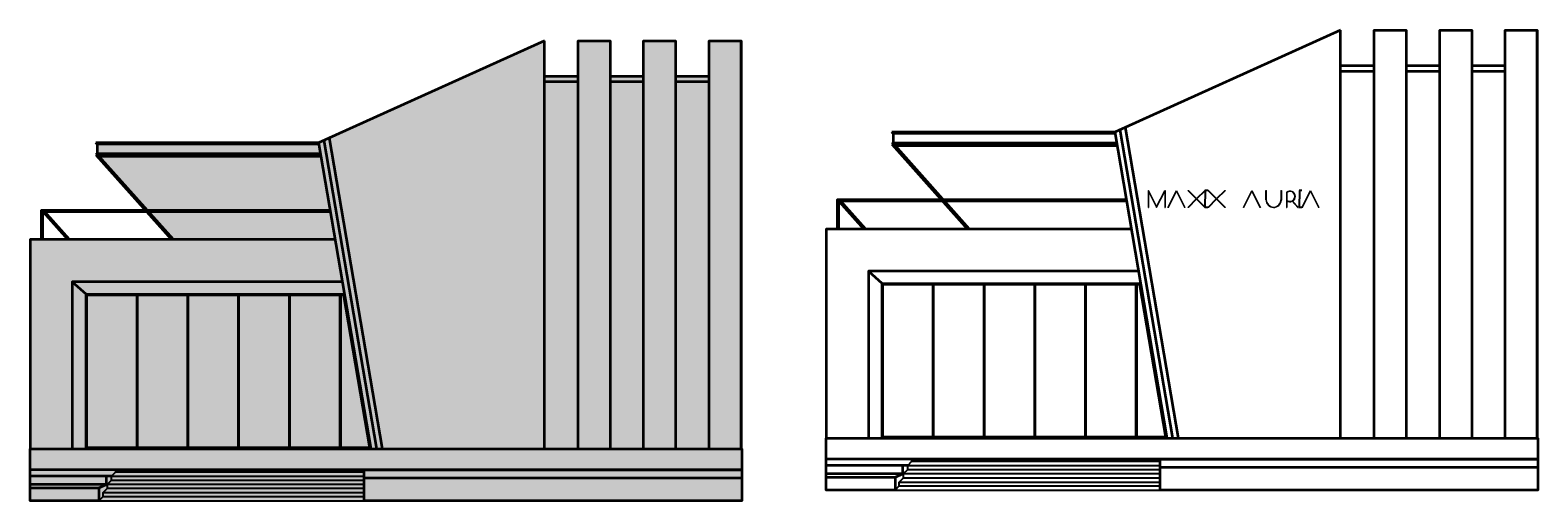
# Model space of a CAD drawing. Units: feet. Extents: x 2182 to 4044, y 1337 to 1918.
import ezdxf

# ---------------------------------------------------------------- set-up
doc = ezdxf.new("R2010")
doc.units = ezdxf.units.FT
for name, color, linetype, lineweight in [('A-ANNO-DIMS', 2, 'Continuous', 18), ('A-ELEV', 7, 'Continuous', 35), ('A-ELEV-PATT', 8, 'Continuous', 13), ('A-ELEV-SIGN', 2, 'Continuous', 18), ('A-FLOR-STRS', 3, 'Continuous', 25), ('A-GLAZ', 4, 'Continuous', 25)]:
    doc.layers.add(name, color=color, linetype=linetype, lineweight=lineweight)
doc.styles.get("Standard").update_dxf_attribs({"font": 'arial.ttf'})
doc.dimstyles.get("Standard").update_dxf_attribs({"dimtxt": 0.18, "dimasz": 0.18, "dimexe": 0.18, "dimexo": 0.0625, "dimgap": 0.09, "dimtad": 0, "dimtih": 1, "dimtoh": 1, "dimdec": 1, "dimzin": 0, "dimdsep": 46, "dimlunit": 3, "dimtxsty": 'Standard', "dimcen": 0.09, "dimadec": 0, "dimazin": 0, "dimtfac": 1, "dimtdec": 1, "dimtofl": 0, "dimtmove": 0, "dimatfit": 3, "dimfxl": 1, "dimtolj": 1, "dimtzin": 0, "dimarcsym": 0})

# ---------------------------------------------------------------- blocks, each defined once
blk = doc.blocks.new('B2')
for p, q in [((0, 21), (10.5, 10.5)), ((0.8, 21), (10.9, 10.9)), ((21, 21), (10.9, 10.9)), ((21.8, 21), (11.3, 10.5)), ((21, 21), (21.8, 21)), ((10.5, 10.5), (0, 0)), ((10.9, 10.1), (0.8, 0)), ((10.9, 10.1), (21, 0)), ((11.3, 10.5), (21.8, 0)), ((21, 0), (21.8, 0))]:
    blk.add_line(p, q)
for points in [[(0, 21), (0.8, 21)], [(0.8, 0), (0, 0)]]:
    blk.add_lwpolyline(points)
blk = doc.blocks.new('B1')
for p, q in [((0, 0), (10.5, 21)), ((0.6, 0), (10.5, 19.8)), ((10.5, 21), (21, 0)), ((10.5, 19.8), (20.4, 0))]:
    blk.add_line(p, q)
for points in [[(0.6, 0), (0, 0)], [(21, 0), (20.4, 0)]]:
    blk.add_lwpolyline(points)
blk = doc.blocks.new('*D4')
at = {"layer": 'A-ANNO-DIMS', "color": 0, "lineweight": -2, "transparency": 16777216}
for p, q in [((3752.6, 1720), (3749.3, 1720)), ((3749.5, 1719.8), (3749.5, 1709.7)), ((3752.6, 1699), (3749.3, 1699)), ((3749.5, 1699.2), (3749.5, 1709.3))]:
    blk.add_line(p, q, dxfattribs=at)
at = {"layer": 'A-ANNO-DIMS', "color": 0, "transparency": 16777216}
for points in [[(3749.5, 1719.8), (3749.5, 1719.8), (3749.5, 1720)], [(3749.5, 1699.2), (3749.5, 1699.2), (3749.5, 1699)]]:
    blk.add_solid(points, dxfattribs=at)
at = {"layer": 'Defpoints', "color": 0, "transparency": 16777216}
for p in [(3749.5, 1720), (3752.6, 1720), (3752.6, 1699)]:
    blk.add_point(p, dxfattribs=at)
at = {"layer": 'A-ANNO-DIMS', "color": 0, "transparency": 16777216, "insert": (3749.5, 1709.5), "char_height": 0.18, "attachment_point": 5}
blk.add_mtext('\\A1;21 TYP.', dxfattribs=at)
blk = doc.blocks.new('*D6')
at = {"layer": 'A-ANNO-DIMS', "color": 0, "lineweight": -2, "transparency": 16777216}
for p, q in [((3636.3, 1720), (3632.9, 1720)), ((3633.1, 1719.8), (3633.1, 1709.7)), ((3636.3, 1699), (3632.9, 1699)), ((3633.1, 1699.2), (3633.1, 1709.3))]:
    blk.add_line(p, q, dxfattribs=at)
at = {"layer": 'A-ANNO-DIMS', "color": 0, "transparency": 16777216}
for points in [[(3633.1, 1719.8), (3633.1, 1719.8), (3633.1, 1720)], [(3633.1, 1699.2), (3633.1, 1699.2), (3633.1, 1699)]]:
    blk.add_solid(points, dxfattribs=at)
at = {"layer": 'Defpoints', "color": 0, "transparency": 16777216}
for p in [(3636.4, 1720), (3633.1, 1699), (3636.4, 1699)]:
    blk.add_point(p, dxfattribs=at)
at = {"layer": 'A-ANNO-DIMS', "color": 0, "transparency": 16777216, "insert": (3633.1, 1709.5), "char_height": 0.18, "attachment_point": 5}
blk.add_mtext('\\A1;21 TYP.', dxfattribs=at)

msp = doc.modelspace()

# ---------------------------------------------------------------- hatches: boundary and pattern name
at = {"layer": 'A-ELEV-PATT'}
h = msp.add_hatch(color=256, dxfattribs=at)
h.dxf.hatch_style = 1
h.paths.add_polyline_path([(2817, 1904.9), (2550.9, 1784.7), (2616.4, 1400.9), (2817, 1400.9)])
h.paths.add_polyline_path([(2979, 1904.9), (2939.5, 1904.9), (2939.5, 1400.9), (2979, 1400.9)])
h.paths.add_polyline_path([(3060, 1904.9), (3020.5, 1904.9), (3020.5, 1400.9), (3060, 1400.9)])
h.paths.add_polyline_path([(2898, 1904.9), (2858.5, 1904.9), (2858.5, 1400.9), (2898, 1400.9)])
h.paths.add_polyline_path([(2233.7, 1607.2), (2567.3, 1607.2), (2558.4, 1659.3), (2197.3, 1659.3), (2181.6, 1659.3), (2181.6, 1400.9), (2233.7, 1400.9)])
h.paths.add_polyline_path([(2266.6, 1353), (2181.6, 1353), (2181.6, 1336.7), (2266.6, 1336.7)])
h.paths.add_polyline_path([(2277.1, 1352.2), (2277.1, 1357.2), (2282.3, 1362.4), (2282.3, 1367.4), (2276.1, 1367.4), (2276.1, 1356.8), (2266.6, 1353), (2266.6, 1336.7), (2271.9, 1342), (2271.9, 1347)])
h.paths.add_polyline_path([(2594.1, 1375.1), (2287.5, 1375.1), (2287.5, 1372.6), (2594.1, 1372.6)])
h.paths.add_polyline_path([(2594.1, 1372.6), (2287.5, 1372.6), (2282.3, 1367.4), (2594.1, 1367.4)])
h.paths.add_polyline_path([(2594.1, 1367.4), (2282.3, 1367.4), (2282.3, 1362.4), (2594.1, 1362.4)])
h.paths.add_polyline_path([(2594.1, 1362.4), (2282.3, 1362.4), (2277.1, 1357.2), (2594.1, 1357.2)])
h.paths.add_polyline_path([(2594.1, 1357.2), (2277.1, 1357.2), (2277.1, 1352.2), (2594.1, 1352.2)])
h.paths.add_polyline_path([(2594.1, 1352.2), (2277.1, 1352.2), (2271.9, 1347), (2594.1, 1347)])
h.paths.add_polyline_path([(2594.1, 1347), (2271.9, 1347), (2271.9, 1342), (2594.1, 1342)])
h.paths.add_polyline_path([(2594.1, 1342), (2271.9, 1342), (2266.6, 1336.7), (2594.1, 1336.7)])
h.paths.add_polyline_path([(3060.7, 1400.9), (2181.6, 1400.9), (2181.6, 1375.1), (3060.7, 1375.1)])
h = msp.add_hatch(color=256, dxfattribs=at)
h.paths.add_polyline_path([(3020.5, 1861.3), (2979, 1861.3), (2979, 1854.5), (3020.5, 1854.5)])
h.paths.add_polyline_path([(2939.5, 1861.3), (2898, 1861.3), (2898, 1854.5), (2939.5, 1854.5)])
h.paths.add_polyline_path([(2858.5, 1861.3), (2817, 1861.3), (2817, 1854.5), (2858.5, 1854.5)])
h.paths.add_polyline_path([(2538, 1778.9), (2262.8, 1778.9), (2264.5, 1777.2), (2538.3, 1777.2)])
h.paths.add_polyline_path([(2538.3, 1777.2), (2264.5, 1777.2), (2264.5, 1765.8), (2540.2, 1765.8)])
h.paths.add_polyline_path([(2540.2, 1765.8), (2264.5, 1765.8), (2262.8, 1764.1), (2540.5, 1764.1)])
h.paths.add_polyline_path([(2540.5, 1764.1), (2262.8, 1764.1), (2264.3, 1762.4), (2412.3, 1762.4), (2540.8, 1762.4)])
h.paths.add_polyline_path([(2266.6, 1762.4), (2264.3, 1762.4), (2323.8, 1695.8), (2326, 1695.8)])
h.paths.add_polyline_path([(2323.8, 1695.8), (2195.6, 1695.8), (2195.6, 1659.3), (2197.3, 1659.3), (2197.3, 1693.9), (2228.2, 1659.3), (2230.4, 1659.3), (2199.4, 1694.1), (2325.3, 1694.1)])
h.paths.add_polyline_path([(2552.1, 1695.8), (2326, 1695.8), (2327.5, 1694.1), (2552.4, 1694.1)])
h.paths.add_polyline_path([(2326, 1695.8), (2323.8, 1695.8), (2325.3, 1694.1), (2327.5, 1694.1)])
h.paths.add_polyline_path([(2327.5, 1694.1), (2325.3, 1694.1), (2356.3, 1659.3), (2358.6, 1659.3)])
h.paths.add_polyline_path([(2569.8, 1592.4), (2250.3, 1592.4), (2250.3, 1400.9), (2602.5, 1400.9)])
h.paths.add_polyline_path([(2314.7, 1590.8), (2375.7, 1590.8), (2375.7, 1402.6), (2314.7, 1402.6)], flags=16)
h.paths.add_polyline_path([(2313, 1402.6), (2252, 1402.6), (2252, 1590.8), (2313, 1590.8)], flags=16)
h.paths.add_polyline_path([(2377.3, 1590.8), (2438.3, 1590.8), (2438.3, 1402.6), (2377.3, 1402.6)], flags=16)
h.paths.add_polyline_path([(2440, 1590.8), (2501, 1590.8), (2501, 1402.6), (2440, 1402.6)], flags=16)
h.paths.add_polyline_path([(2502.7, 1590.8), (2563.7, 1590.8), (2563.7, 1402.6), (2502.7, 1402.6)], flags=16)
h.paths.add_polyline_path([(2565.4, 1590.8), (2568.4, 1590.8), (2600.5, 1402.6), (2565.4, 1402.6)], flags=16)
h = msp.add_hatch(color=256, dxfattribs=at)
h.paths.add_polyline_path([(2858.5, 1854.5), (2817, 1854.5), (2817, 1400.9), (2858.5, 1400.9)])
h.paths.add_polyline_path([(2939.5, 1854.5), (2898, 1854.5), (2898, 1400.9), (2939.5, 1400.9)])
h.paths.add_polyline_path([(3020.5, 1854.5), (2979, 1854.5), (2979, 1400.9), (3020.5, 1400.9)])
h.paths.add_polyline_path([(2313, 1590.8), (2252, 1590.8), (2252, 1402.6), (2313, 1402.6)])
h.paths.add_polyline_path([(2375.7, 1590.8), (2314.7, 1590.8), (2314.7, 1402.6), (2375.7, 1402.6)])
h.paths.add_polyline_path([(2438.3, 1590.8), (2377.3, 1590.8), (2377.3, 1402.6), (2438.3, 1402.6)])
h.paths.add_polyline_path([(2501, 1590.8), (2440, 1590.8), (2440, 1402.6), (2501, 1402.6)])
h.paths.add_polyline_path([(2563.7, 1590.8), (2502.7, 1590.8), (2502.7, 1402.6), (2563.7, 1402.6)])
h.paths.add_polyline_path([(2568.4, 1590.8), (2565.4, 1590.8), (2565.4, 1402.6), (2600.5, 1402.6)])
for points in [[(2544.4, 1781.8), (2538, 1778.9), (2602.5, 1400.9), (2609.5, 1400.9)], [(2550.9, 1784.7), (2544.4, 1781.8), (2609.5, 1400.9), (2616.4, 1400.9)]]:
    msp.add_hatch(color=256, dxfattribs=at).paths.add_polyline_path(points)
h = msp.add_hatch(color=256, dxfattribs=at)
h.paths.add_polyline_path([(2540.8, 1762.4), (2266.6, 1762.4), (2326, 1695.8), (2552.1, 1695.8)])
h.paths.add_polyline_path([(2552.4, 1694.1), (2327.5, 1694.1), (2358.6, 1659.3), (2558.4, 1659.3)])
h = msp.add_hatch(color=256, dxfattribs=at)
h.paths.add_polyline_path([(2579.8, 1705.8), (2589.7, 1685.9), (2599.7, 1705.8), (2599.7, 1685.9), (2600.2, 1685.9), (2600.2, 1706.9), (2599.7, 1706.9), (2589.7, 1687), (2579.8, 1706.9), (2579.2, 1706.9), (2579.2, 1685.9), (2579.8, 1685.9)])
h.paths.add_polyline_path([(2614.3, 1705.7), (2624.2, 1685.9), (2624.8, 1685.9), (2614.3, 1706.9), (2603.8, 1685.9), (2604.4, 1685.9)])
h.paths.add_polyline_path([(2650, 1706.9), (2649.1, 1706.9), (2639, 1696.8), (2629, 1706.9), (2628.1, 1706.9), (2638.6, 1696.4), (2628.1, 1685.9), (2629, 1685.9), (2639, 1696), (2649.1, 1685.9), (2650, 1685.9), (2639.5, 1696.4)])
h.paths.add_polyline_path([(2674.8, 1706.9), (2673.9, 1706.9), (2663.8, 1696.8), (2653.7, 1706.9), (2652.9, 1706.9), (2663.4, 1696.4), (2652.9, 1685.9), (2653.7, 1685.9), (2663.8, 1696), (2673.9, 1685.9), (2674.8, 1685.9), (2664.2, 1696.4)])
h.paths.add_polyline_path([(2707.4, 1706.9), (2696.9, 1685.9), (2697.5, 1685.9), (2707.4, 1705.7), (2717.3, 1685.9), (2717.9, 1685.9)])
h.paths.add_polyline_path([(2725.3, 1695.5), (2725.3, 1706.9), (2724.7, 1706.9), (2724.7, 1695.5, 0.971712), (2743.9, 1695), (2743.9, 1706.9), (2743.3, 1706.9), (2743.3, 1695.5, -1)])
h.paths.add_polyline_path([(2750.3, 1704.8), (2750.3, 1685.9), (2750.8, 1685.9), (2750.8, 1694, 0.253815), (2757.1, 1693.5), (2764.3, 1685.9), (2765.1, 1685.9), (2757.7, 1693.8, 1.091288)])
h.paths.add_polyline_path([(2750.8, 1694.7), (2750.8, 1704.5, -1.982009)], flags=16)
h.paths.add_polyline_path([(2779.7, 1705.7), (2789.6, 1685.9), (2790.2, 1685.9), (2779.7, 1706.9), (2769.2, 1685.9), (2769.8, 1685.9)])
h = msp.add_hatch(color=256, dxfattribs=at)
h.paths.add_polyline_path([(2250.3, 1592.4), (2233.7, 1607.2), (2233.7, 1400.9), (2250.3, 1400.9)])
h.paths.add_polyline_path([(2567.3, 1607.2), (2233.7, 1607.2), (2250.3, 1592.4), (2569.8, 1592.4)])
h = msp.add_hatch(color=256, dxfattribs=at)
h.set_gradient(color1=(19, 155, 72), color2=(19, 155, 72), tint=1)
h.paths.add_polyline_path([(2276.1, 1356.8), (2181.6, 1356.8), (2181.6, 1353), (2266.6, 1353)])
h.paths.add_polyline_path([(2287.5, 1372.6), (2287.5, 1375.1), (2181.6, 1375.1), (2181.6, 1367.4), (2282.3, 1367.4)])
h.paths.add_polyline_path([(3060.7, 1375.1), (2594.1, 1375.1), (2594.1, 1365.3), (3060.7, 1365.3)])
h = msp.add_hatch(dxfattribs=at)
h.set_pattern_fill('GRASS', color=256, scale=0.1, style=0)
h.paths.add_polyline_path([(2287.5, 1372.6), (2287.5, 1375.1), (2181.6, 1375.1), (2181.6, 1367.4), (2282.3, 1367.4)])
h.paths.add_polyline_path([(2276.1, 1356.8), (2181.6, 1356.8), (2181.6, 1353), (2266.6, 1353)])
h.paths.add_polyline_path([(3060.7, 1375.1), (2594.1, 1375.1), (2594.1, 1365.3), (3060.7, 1365.3)])
h = msp.add_hatch(color=256, dxfattribs=at)
h.dxf.hatch_style = 1
h.paths.add_polyline_path([(2276.1, 1367.4), (2181.6, 1367.4), (2181.6, 1356.8), (2276.1, 1356.8)])
h = msp.add_hatch(color=256, dxfattribs=at)
h.dxf.hatch_style = 1
h.paths.add_polyline_path([(3060.7, 1365.3), (2594.1, 1365.3), (2594.1, 1336.7), (3060.7, 1336.7)])

# ---------------------------------------------------------------- linework, layer by layer
at = {"layer": 'A-ELEV'}
for p, q in [((2817, 1904.9), (2538, 1778.9)), ((2817, 1904.9), (2538, 1778.9)), ((2817, 1400.9), (2817, 1904.9)), ((2817, 1400.9), (2817, 1904.9)), ((3060, 1400.9), (3060, 1904.9)), ((3060, 1898.9), (3060, 1904.9)), ((3060, 1400.9), (3060, 1904.9)), ((3060, 1898.9), (3060, 1904.9)), ((3800.4, 1918), (3521.4, 1792)), ((3800.4, 1414), (3800.4, 1918)), ((4043.4, 1414), (4043.4, 1918)), ((4043.4, 1912), (4043.4, 1918)), ((3800.4, 1874.4), (3841.9, 1874.4)), ((3800.4, 1867.5), (3841.9, 1867.5)), ((3881.4, 1874.4), (3922.9, 1874.4)), ((3881.4, 1867.5), (3922.9, 1867.5)), ((3962.4, 1874.4), (4003.9, 1874.4)), ((3962.4, 1867.5), (4003.9, 1867.5)), ((2817, 1861.3), (2858.5, 1861.3)), ((2817, 1861.3), (2858.5, 1861.3)), ((2817, 1854.5), (2858.5, 1854.5)), ((2817, 1854.5), (2858.5, 1854.5)), ((2898, 1861.3), (2939.5, 1861.3)), ((2898, 1861.3), (2939.5, 1861.3)), ((2898, 1854.5), (2939.5, 1854.5)), ((2898, 1854.5), (2939.5, 1854.5)), ((2979, 1861.3), (3020.5, 1861.3)), ((2979, 1861.3), (3020.5, 1861.3)), ((2979, 1854.5), (3020.5, 1854.5)), ((2979, 1854.5), (3020.5, 1854.5)), ((3247.9, 1790.3), (3246.2, 1792)), ((3521.4, 1792), (3585.9, 1414)), ((3527.8, 1794.9), (3592.9, 1414)), ((3534.3, 1797.8), (3599.8, 1414)), ((4043.4, 1786), (4043.4, 1792)), ((2264.5, 1777.2), (2262.8, 1778.9)), ((2264.5, 1777.2), (2262.8, 1778.9)), ((2538, 1778.9), (2602.5, 1400.9)), ((2538, 1778.9), (2602.5, 1400.9)), ((2544.4, 1781.8), (2609.5, 1400.9)), ((2544.4, 1781.8), (2609.5, 1400.9)), ((2550.9, 1784.7), (2616.4, 1400.9)), ((2550.9, 1784.7), (2616.4, 1400.9)), ((3060, 1772.9), (3060, 1778.9)), ((3060, 1772.9), (3060, 1778.9)), ((3247.9, 1778.9), (3246.2, 1777.2)), ((3246.2, 1777.2), (3339.7, 1672.4)), ((2264.5, 1765.8), (2262.8, 1764.1)), ((2264.5, 1765.8), (2262.8, 1764.1)), ((2262.8, 1764.1), (2356.3, 1659.3)), ((2262.8, 1764.1), (2356.3, 1659.3)), ((3180.7, 1707), (3211.6, 1672.4)), ((2197.3, 1693.9), (2228.2, 1659.3)), ((2197.3, 1693.9), (2228.2, 1659.3)), ((4043.4, 1660), (4043.4, 1666)), ((3060, 1646.9), (3060, 1652.9)), ((3060, 1646.9), (3060, 1652.9)), ((2233.7, 1607.2), (2250.3, 1592.4)), ((2233.7, 1607.2), (2250.3, 1592.4)), ((3217.1, 1620.3), (3233.7, 1605.5)), ((3233.7, 1605.5), (3233.7, 1414)), ((2250.3, 1592.4), (2250.3, 1400.9)), ((2250.3, 1592.4), (2250.3, 1400.9)), ((4043.4, 1534), (4043.4, 1540)), ((3060, 1520.9), (3060, 1526.9)), ((3060, 1520.9), (3060, 1526.9)), ((2181.6, 1400.9), (3060, 1400.9)), ((2181.6, 1400.9), (3060, 1400.9)), ((3165, 1414), (4043.4, 1414)), ((3265.7, 1380.5), (3165, 1380.5)), ((3259.5, 1369.9), (3259.5, 1380.5)), ((3577.5, 1378.4), (4044.1, 1378.4)), ((2282.3, 1367.4), (2181.6, 1367.4)), ((2282.3, 1367.4), (2181.6, 1367.4)), ((2276.1, 1356.8), (2276.1, 1367.4)), ((2276.1, 1356.8), (2276.1, 1367.4)), ((2594.1, 1365.3), (3060.7, 1365.3)), ((2594.1, 1365.3), (3060.7, 1365.3)), ((3259.5, 1369.9), (3165, 1369.9)), ((3165, 1366.1), (3250, 1366.1)), ((3250, 1366.1), (3259.5, 1369.9)), ((3250, 1366.1), (3250, 1349.8)), ((2276.1, 1356.8), (2181.6, 1356.8)), ((2276.1, 1356.8), (2181.6, 1356.8)), ((2181.6, 1353), (2266.6, 1353)), ((2181.6, 1353), (2266.6, 1353)), ((2266.6, 1353), (2276.1, 1356.8)), ((2266.6, 1353), (2276.1, 1356.8)), ((2266.6, 1353), (2266.6, 1336.7)), ((2266.6, 1353), (2266.6, 1336.7))]:
    msp.add_line(p, q, dxfattribs=at)
for points in [[(2858.5, 1400.9), (2858.5, 1904.9), (2898, 1904.9), (2898, 1400.9)], [(2858.5, 1400.9), (2858.5, 1904.9), (2898, 1904.9), (2898, 1400.9)], [(2939.5, 1400.9), (2939.5, 1904.9), (2979, 1904.9), (2979, 1400.9)], [(2939.5, 1400.9), (2939.5, 1904.9), (2979, 1904.9), (2979, 1400.9)], [(3020.5, 1400.9), (3020.5, 1904.9), (3060, 1904.9), (3060, 1400.9)], [(3020.5, 1400.9), (3020.5, 1904.9), (3060, 1904.9), (3060, 1400.9)], [(3841.9, 1414), (3841.9, 1918), (3881.4, 1918), (3881.4, 1414)], [(3922.9, 1414), (3922.9, 1918), (3962.4, 1918), (3962.4, 1414)], [(4003.9, 1414), (4003.9, 1918), (4043.4, 1918), (4043.4, 1414)], [(3521.4, 1792), (3246.2, 1792)], [(3521.7, 1790.3), (3247.9, 1790.3), (3247.9, 1778.9), (3523.6, 1778.9)], [(2538, 1778.9), (2262.8, 1778.9)], [(2538, 1778.9), (2262.8, 1778.9)], [(2538.3, 1777.2), (2264.5, 1777.2), (2264.5, 1765.8), (2540.2, 1765.8)], [(2538.3, 1777.2), (2264.5, 1777.2), (2264.5, 1765.8), (2540.2, 1765.8)], [(3246.2, 1777.2), (3523.9, 1777.2)], [(3247.7, 1775.5), (3395.8, 1775.5)], [(3342, 1672.4), (3250, 1775.5), (3524.2, 1775.5)], [(2262.8, 1764.1), (2540.5, 1764.1)], [(2262.8, 1764.1), (2540.5, 1764.1)], [(2264.3, 1762.4), (2412.3, 1762.4)], [(2264.3, 1762.4), (2412.3, 1762.4)], [(2358.6, 1659.3), (2266.6, 1762.4), (2540.8, 1762.4)], [(2358.6, 1659.3), (2266.6, 1762.4), (2540.8, 1762.4)], [(2195.6, 1659.3), (2195.6, 1695.8), (2552.1, 1695.8)], [(2195.6, 1659.3), (2195.6, 1695.8), (2552.1, 1695.8)], [(3179, 1672.4), (3179, 1708.9), (3535.6, 1708.9)], [(3541.8, 1672.4), (3180.7, 1672.4), (3180.7, 1707)], [(3182.8, 1707.2), (3535.8, 1707.2)], [(3213.9, 1672.4), (3182.8, 1707.2)], [(2558.4, 1659.3), (2197.3, 1659.3), (2197.3, 1693.9)], [(2558.4, 1659.3), (2197.3, 1659.3), (2197.3, 1693.9)], [(2230.4, 1659.3), (2199.4, 1694.1)], [(2199.4, 1694.1), (2552.4, 1694.1)], [(2199.4, 1694.1), (2552.4, 1694.1)], [(2230.4, 1659.3), (2199.4, 1694.1)], [(2558.4, 1659.3), (2181.6, 1659.3), (2181.6, 1400.9)], [(2558.4, 1659.3), (2181.6, 1659.3), (2181.6, 1400.9)], [(3541.8, 1672.4), (3165, 1672.4), (3165, 1414)], [(2567.3, 1607.2), (2233.7, 1607.2), (2233.7, 1400.9)], [(2567.3, 1607.2), (2233.7, 1607.2), (2233.7, 1400.9)], [(3550.7, 1620.3), (3217.1, 1620.3), (3217.1, 1414)], [(3250, 1349.8), (3165, 1349.8), (3165, 1388.2)], [(2266.6, 1336.7), (2181.6, 1336.7), (2181.6, 1375.1)], [(2266.6, 1336.7), (2181.6, 1336.7), (2181.6, 1375.1)]]:
    msp.add_lwpolyline(points, dxfattribs=at)
for points in [[(2181.6, 1400.9), (3060.7, 1400.9), (3060.7, 1375.1), (2181.6, 1375.1)], [(2181.6, 1400.9), (3060.7, 1400.9), (3060.7, 1375.1), (2181.6, 1375.1)], [(3165, 1414), (4044.1, 1414), (4044.1, 1388.2), (3165, 1388.2)], [(3577.5, 1388.2), (4044.1, 1388.2), (4044.1, 1349.8), (3577.5, 1349.8)], [(2594.1, 1375.1), (3060.7, 1375.1), (3060.7, 1336.7), (2594.1, 1336.7)], [(2594.1, 1375.1), (3060.7, 1375.1), (3060.7, 1336.7), (2594.1, 1336.7)]]:
    msp.add_lwpolyline(points, close=True, dxfattribs=at)
at = {"layer": 'A-ELEV-SIGN'}
for p, q in [((3562.7, 1720), (3562.7, 1699)), ((3562.7, 1720), (3563.2, 1720)), ((3563.2, 1718.9), (3563.2, 1699)), ((3583.1, 1720), (3583.7, 1720)), ((3583.1, 1718.9), (3583.1, 1699)), ((3583.7, 1720), (3583.7, 1699)), ((3733.7, 1717.9), (3733.7, 1699)), ((3734.2, 1717.6), (3734.2, 1707.8)), ((3562.7, 1699), (3563.2, 1699)), ((3583.1, 1699), (3583.7, 1699)), ((3733.7, 1699), (3734.2, 1699)), ((3734.2, 1707.1), (3734.2, 1699)), ((3740.5, 1706.6), (3747.7, 1699)), ((3741.1, 1706.9), (3748.5, 1699)), ((3747.7, 1699), (3748.5, 1699))]:
    msp.add_line(p, q, dxfattribs=at)
for points in [[(3563.2, 1720), (3573.2, 1700.1), (3583.1, 1720)], [(3563.2, 1718.9), (3573.2, 1699), (3583.1, 1718.9)], [(3708.1, 1708.6), (3708.1, 1720)], [(3708.1, 1720), (3708.7, 1720)], [(3708.7, 1708.6), (3708.7, 1720)], [(3726.7, 1720), (3726.7, 1708.6)], [(3726.7, 1720), (3727.3, 1720)], [(3727.3, 1720), (3727.3, 1708)]]:
    msp.add_lwpolyline(points, dxfattribs=at)
for centre, radius, start, end in [((3737.9, 1712.7), 6.65, 298.883, 128.8808), ((3737.9, 1712.7), 6.1, 233.5454, 126.4546), ((3717.7, 1708.6), 9.58, 180, 356.7122), ((3717.7, 1708.6), 9.03, 180, 0), ((3737.9, 1712.7), 6.65, 236.9678, 293.9349)]:
    msp.add_arc(centre, radius, start, end, dxfattribs=at)
at = {"layer": 'A-FLOR-STRS'}
for p, q in [((3265.7, 1380.5), (3577.5, 1380.5)), ((3270.9, 1385.7), (3577.5, 1385.7)), ((2282.3, 1367.4), (2594.1, 1367.4)), ((2282.3, 1367.4), (2594.1, 1367.4)), ((2282.3, 1362.4), (2594.1, 1362.4)), ((2282.3, 1362.4), (2594.1, 1362.4)), ((2287.5, 1372.6), (2594.1, 1372.6)), ((2287.5, 1372.6), (2594.1, 1372.6)), ((3255.3, 1360), (3577.5, 1360)), ((3260.5, 1370.3), (3577.5, 1370.3)), ((3260.5, 1365.3), (3577.5, 1365.3)), ((3265.7, 1375.5), (3577.5, 1375.5)), ((2271.9, 1347), (2594.1, 1347)), ((2271.9, 1347), (2594.1, 1347)), ((2271.9, 1342), (2594.1, 1342)), ((2271.9, 1342), (2594.1, 1342)), ((2277.1, 1357.2), (2594.1, 1357.2)), ((2277.1, 1357.2), (2594.1, 1357.2)), ((2277.1, 1352.2), (2594.1, 1352.2)), ((2277.1, 1352.2), (2594.1, 1352.2)), ((3250, 1349.8), (3577.5, 1349.8)), ((3255.3, 1355.1), (3577.5, 1355.1)), ((2266.6, 1336.7), (2594.1, 1336.7)), ((2266.6, 1336.7), (2594.1, 1336.7))]:
    msp.add_line(p, q, dxfattribs=at)
for points in [[(3260.5, 1370.3), (3265.7, 1375.5), (3265.7, 1380.5)], [(3265.7, 1380.5), (3270.9, 1385.7), (3270.9, 1388.2)], [(2277.1, 1357.2), (2282.3, 1362.4), (2282.3, 1367.4)], [(2277.1, 1357.2), (2282.3, 1362.4), (2282.3, 1367.4)], [(2282.3, 1367.4), (2287.5, 1372.6), (2287.5, 1375.1)], [(2282.3, 1367.4), (2287.5, 1372.6), (2287.5, 1375.1)], [(3250, 1349.8), (3255.3, 1355.1), (3255.3, 1360)], [(3255.3, 1360), (3260.5, 1365.3), (3260.5, 1370.3)], [(2266.6, 1336.7), (2271.9, 1342), (2271.9, 1347)], [(2266.6, 1336.7), (2271.9, 1342), (2271.9, 1347)], [(2271.9, 1347), (2277.1, 1352.2), (2277.1, 1357.2)], [(2271.9, 1347), (2277.1, 1352.2), (2277.1, 1357.2)]]:
    msp.add_lwpolyline(points, dxfattribs=at)
at = {"layer": 'A-GLAZ'}
for p, q in [((3548.8, 1603.9), (3548.8, 1415.7)), ((3551.8, 1603.9), (3583.9, 1415.7)), ((2565.4, 1590.8), (2565.4, 1402.6)), ((2565.4, 1590.8), (2565.4, 1402.6)), ((2568.4, 1590.8), (2600.5, 1402.6)), ((2568.4, 1590.8), (2600.5, 1402.6))]:
    msp.add_line(p, q, dxfattribs=at)
for points in [[(3585.9, 1414), (3233.7, 1414), (3233.7, 1605.5), (3553.2, 1605.5)], [(3548.8, 1603.9), (3551.8, 1603.9)], [(2602.5, 1400.9), (2250.3, 1400.9), (2250.3, 1592.4), (2569.8, 1592.4)], [(2602.5, 1400.9), (2250.3, 1400.9), (2250.3, 1592.4), (2569.8, 1592.4)], [(2565.4, 1590.8), (2568.4, 1590.8)], [(2565.4, 1590.8), (2568.4, 1590.8)], [(3583.9, 1415.7), (3548.8, 1415.7)], [(2600.5, 1402.6), (2565.4, 1402.6)], [(2600.5, 1402.6), (2565.4, 1402.6)]]:
    msp.add_lwpolyline(points, dxfattribs=at)
for points in [[(3296.4, 1415.7), (3235.4, 1415.7), (3235.4, 1603.9), (3296.4, 1603.9)], [(3298.1, 1415.7), (3298.1, 1603.9), (3359.1, 1603.9), (3359.1, 1415.7)], [(3360.8, 1415.7), (3360.8, 1603.9), (3421.7, 1603.9), (3421.7, 1415.7)], [(3423.4, 1415.7), (3423.4, 1603.9), (3484.4, 1603.9), (3484.4, 1415.7)], [(3486.1, 1415.7), (3486.1, 1603.9), (3547.1, 1603.9), (3547.1, 1415.7)], [(2313, 1402.6), (2252, 1402.6), (2252, 1590.8), (2313, 1590.8)], [(2313, 1402.6), (2252, 1402.6), (2252, 1590.8), (2313, 1590.8)], [(2314.7, 1402.6), (2314.7, 1590.8), (2375.7, 1590.8), (2375.7, 1402.6)], [(2314.7, 1402.6), (2314.7, 1590.8), (2375.7, 1590.8), (2375.7, 1402.6)], [(2377.3, 1402.6), (2377.3, 1590.8), (2438.3, 1590.8), (2438.3, 1402.6)], [(2377.3, 1402.6), (2377.3, 1590.8), (2438.3, 1590.8), (2438.3, 1402.6)], [(2440, 1402.6), (2440, 1590.8), (2501, 1590.8), (2501, 1402.6)], [(2440, 1402.6), (2440, 1590.8), (2501, 1590.8), (2501, 1402.6)], [(2502.7, 1402.6), (2502.7, 1590.8), (2563.7, 1590.8), (2563.7, 1402.6)], [(2502.7, 1402.6), (2502.7, 1590.8), (2563.7, 1590.8), (2563.7, 1402.6)]]:
    msp.add_lwpolyline(points, close=True, dxfattribs=at)

# ---------------------------------------------------------------- block references
at = {"layer": 'A-ELEV-SIGN'}
for name, p in [('B1', (3587.2, 1699)), ('B2', (3611.6, 1699)), ('B1', (3680.3, 1699)), ('B1', (3752.6, 1699))]:
    msp.add_blockref(name, p, dxfattribs=at)
at = {"layer": 'A-ELEV-SIGN', "rotation": 180}
msp.add_blockref('B2', (3658.2, 1720), dxfattribs=at)

# ---------------------------------------------------------------- dimensions: what is measured, and where the dimension line sits
at = {"layer": 'A-ANNO-DIMS'}
for base, p1, p2, angle, picture, middle in [((3633.1, 1699), (3636.4, 1720), (3636.4, 1699), 270, '*D6', (3633.1, 1709.5)), ((3749.5, 1720), (3752.6, 1699), (3752.6, 1720), 90, '*D4', (3749.5, 1709.5))]:
    dim = msp.add_linear_dim(base=base, p1=p1, p2=p2, angle=angle, text='<> TYP.', dimstyle='Standard', override={"dimdec": 0, "dimlfac": 1, "dimrnd": 0, "dimzin": 0, "dimdsep": 46, "dimlunit": 2}, dxfattribs=at)
    dim.commit()
    dim.dimension.update_dxf_attribs({"geometry": picture, "text_midpoint": middle})

doc.saveas('drawing.dxf')
